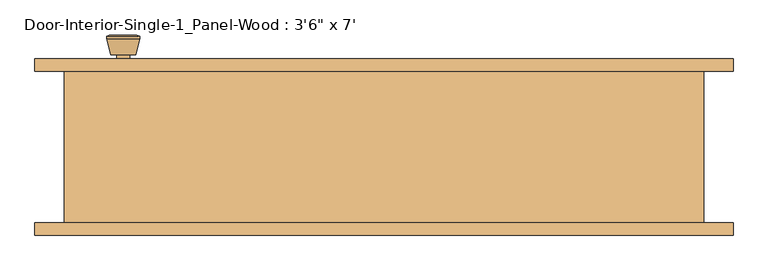
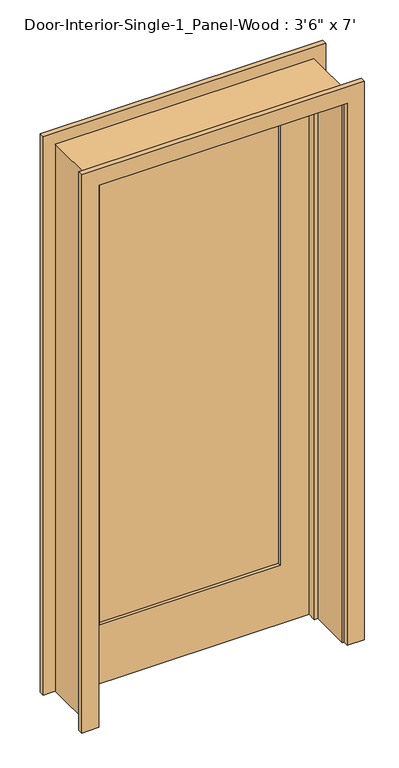
"""IFC4 building model written with IfcOpenShell, lengths in millimetres: door geometry."""

from ifc_helpers import new_model, si_unit, point, frame, frame_2d, origin, place, context, project, spatial, polyline, circle_curve, trimmed, segment, composite_curve, outline, extrude, faceted_brep, source, transform, mapped, element, save
from ifc_brep_helpers import plane_surface, cylinder_surface, revolved_surface, advanced_brep


def door_3b97b8e7(model_context):
    return source(origin(), model_context, "Body", "SolidModel", [
        advanced_brep(
        [(-393.7, 70.2, 914.4), (-383.7, 70.2, 914.4), (-403.7, 70.2, 914.4), (-373.2241324, 21.2, 914.4), (-393.7, 21.2, 914.4), (-414.1758676, 21.2, 914.4), (-368.7, 23.0278681, 914.4), (-418.7, 23.0278681, 914.4), (-368.7, 26.4915463, 914.4), (-418.7, 26.4915463, 914.4), (-375.063764, 51.2, 914.4), (-412.336236, 51.2, 914.4), (-383.7, 51.2, 914.4), (-403.7, 51.2, 914.4)],
        [
            (0, 1),
            (1, 2, circle_curve(frame((-393.7, 70.2, 914.4), z_axis=(0.0, 1.0, 0.0), x_axis=(-1.0, 0.0, 0.0)), 10.0)),
            (2, 0),
            (2, 1, circle_curve(frame((-393.7, 70.2, 914.4), z_axis=(0.0, 1.0, 0.0), x_axis=(-1.0, 0.0, 0.0)), 10.0)),
            (3, 4),
            (4, 5),
            (5, 3, circle_curve(frame((-393.7, 21.2, 914.4), z_axis=(0.0, -1.0, 0.0), x_axis=(-1.0, 0.0, 0.0)), 20.4758676)),
            (3, 5, circle_curve(frame((-393.7, 21.2, 914.4), z_axis=(0.0, -1.0, 0.0), x_axis=(-1.0, 0.0, 0.0)), 20.4758676)),
            (6, 3),
            (5, 7),
            (7, 6, circle_curve(frame((-393.7, 23.0278681, 914.4), z_axis=(0.0, -1.0, 0.0), x_axis=(-1.0, 0.0, 0.0)), 25.0)),
            (6, 7, circle_curve(frame((-393.7, 23.0278681, 914.4), z_axis=(0.0, -1.0, 0.0), x_axis=(-1.0, 0.0, 0.0)), 25.0)),
            (8, 6),
            (7, 9),
            (9, 8, circle_curve(frame((-393.7, 26.4915463, 914.4), z_axis=(0.0, -1.0, 0.0), x_axis=(-1.0, 0.0, 0.0)), 25.0)),
            (8, 9, circle_curve(frame((-393.7, 26.4915463, 914.4), z_axis=(0.0, -1.0, 0.0), x_axis=(-1.0, 0.0, 0.0)), 25.0)),
            (10, 8),
            (9, 11),
            (11, 10, circle_curve(frame((-393.7, 51.2, 914.4), z_axis=(0.0, -1.0, 0.0), x_axis=(-1.0, 0.0, 0.0)), 18.636236)),
            (10, 11, circle_curve(frame((-393.7, 51.2, 914.4), z_axis=(0.0, -1.0, 0.0), x_axis=(-1.0, 0.0, 0.0)), 18.636236)),
            (12, 10),
            (11, 13),
            (13, 12, circle_curve(frame((-393.7, 51.2, 914.4), z_axis=(0.0, -1.0, 0.0), x_axis=(-1.0, 0.0, 0.0)), 10.0)),
            (12, 13, circle_curve(frame((-393.7, 51.2, 914.4), z_axis=(0.0, -1.0, 0.0), x_axis=(-1.0, 0.0, 0.0)), 10.0)),
            (1, 12),
            (13, 2),
        ],
        [
            plane_surface(frame((-393.7, 70.2, 914.4), z_axis=(0.0, 1.0, 0.0), x_axis=(-1.0, 0.0, 0.0))),
            plane_surface(frame((-393.7, 21.2, 914.4), z_axis=(0.0, -1.0, 0.0), x_axis=(-1.0, 0.0, 0.0))),
            revolved_surface(polyline([(-414.1758676, 21.2, 914.4), (-418.7, 23.0278681, 914.4)]), (-393.7, 70.2, 914.4), (0.0, 1.0, 0.0)),
            cylinder_surface(frame((-393.7, 70.2, 914.4), z_axis=(0.0, 1.0, 0.0), x_axis=(-1.0, 0.0, 0.0)), 25.0),
            revolved_surface(polyline([(-418.7, 26.4915463, 914.4), (-412.336236, 51.2, 914.4)]), (-393.7, 70.2, 914.4), (0.0, 1.0, 0.0)),
            plane_surface(frame((-393.7, 51.2, 914.4), z_axis=(0.0, 1.0, 0.0), x_axis=(-1.0, 0.0, 0.0))),
            cylinder_surface(frame((-393.7, 70.2, 914.4), z_axis=(0.0, 1.0, 0.0), x_axis=(-1.0, 0.0, 0.0)), 10.0),
        ],
        [
            (0, [[1, 2, 3]]),
            (0, [[-3, 4, -1]]),
            (1, [[5, 6, 7]]),
            (1, [[-6, -5, 8]]),
            (2, [[9, -7, 10, 11]]),
            (2, [[-10, -8, -9, 12]]),
            (3, [[13, -11, 14, 15]]),
            (3, [[-14, -12, -13, 16]]),
            (4, [[17, -15, 18, 19]]),
            (4, [[-18, -16, -17, 20]]),
            (5, [[21, -19, 22, 23]]),
            (5, [[-22, -20, -21, 24]]),
            (6, [[25, -23, 26, -2]]),
            (6, [[-26, -24, -25, -4]]),
        ],
    ),
        extrude(outline(composite_curve([segment(trimmed(circle_curve(frame_2d((914.4, -393.7)), 30.0), [point((914.4, -423.7))], [point((914.4, -363.7))], False, "CARTESIAN"), True, "CONTINUOUS"), segment(trimmed(circle_curve(frame_2d((914.4, -393.7)), 30.0), [point((914.4, -363.7))], [point((914.4, -423.7))], False, "CARTESIAN"), True, "CONTINUOUS")], self_intersect=False)), frame((0.0, 70.2, 0.0), z_axis=(0.0, 1.0, 0.0), x_axis=(0.0, 0.0, 1.0)), (0.0, 0.0, 1.0), 6.0),
        advanced_brep(
        [(-393.7, 117.125, 914.4), (-403.7, 117.125, 914.4), (-383.7, 117.125, 914.4), (-373.2241324, 166.125, 914.4), (-414.1758676, 166.125, 914.4), (-393.7, 166.125, 914.4), (-368.7, 164.2971319, 914.4), (-418.7, 164.2971319, 914.4), (-368.7, 160.8334537, 914.4), (-418.7, 160.8334537, 914.4), (-375.063764, 136.125, 914.4), (-412.336236, 136.125, 914.4), (-383.7, 136.125, 914.4), (-403.7, 136.125, 914.4)],
        [
            (0, 1),
            (1, 2, circle_curve(frame((-393.7, 117.125, 914.4), z_axis=(0.0, -1.0, 0.0), x_axis=(-1.0, 0.0, 0.0)), 10.0)),
            (2, 0),
            (2, 1, circle_curve(frame((-393.7, 117.125, 914.4), z_axis=(0.0, -1.0, 0.0), x_axis=(-1.0, 0.0, 0.0)), 10.0)),
            (3, 4, circle_curve(frame((-393.7, 166.125, 914.4), z_axis=(0.0, 1.0, 0.0), x_axis=(-1.0, 0.0, 0.0)), 20.4758676)),
            (4, 5),
            (5, 3),
            (4, 3, circle_curve(frame((-393.7, 166.125, 914.4), z_axis=(0.0, 1.0, 0.0), x_axis=(-1.0, 0.0, 0.0)), 20.4758676)),
            (6, 7, circle_curve(frame((-393.7, 164.2971319, 914.4), z_axis=(0.0, 1.0, 0.0), x_axis=(-1.0, 0.0, 0.0)), 25.0)),
            (7, 4),
            (3, 6),
            (7, 6, circle_curve(frame((-393.7, 164.2971319, 914.4), z_axis=(0.0, 1.0, 0.0), x_axis=(-1.0, 0.0, 0.0)), 25.0)),
            (8, 9, circle_curve(frame((-393.7, 160.8334537, 914.4), z_axis=(0.0, 1.0, 0.0), x_axis=(-1.0, 0.0, 0.0)), 25.0)),
            (9, 7),
            (6, 8),
            (9, 8, circle_curve(frame((-393.7, 160.8334537, 914.4), z_axis=(0.0, 1.0, 0.0), x_axis=(-1.0, 0.0, 0.0)), 25.0)),
            (10, 11, circle_curve(frame((-393.7, 136.125, 914.4), z_axis=(0.0, 1.0, 0.0), x_axis=(-1.0, 0.0, 0.0)), 18.636236)),
            (11, 9),
            (8, 10),
            (11, 10, circle_curve(frame((-393.7, 136.125, 914.4), z_axis=(0.0, 1.0, 0.0), x_axis=(-1.0, 0.0, 0.0)), 18.636236)),
            (12, 13, circle_curve(frame((-393.7, 136.125, 914.4), z_axis=(0.0, 1.0, 0.0), x_axis=(-1.0, 0.0, 0.0)), 10.0)),
            (13, 11),
            (10, 12),
            (13, 12, circle_curve(frame((-393.7, 136.125, 914.4), z_axis=(0.0, 1.0, 0.0), x_axis=(-1.0, 0.0, 0.0)), 10.0)),
            (1, 13),
            (12, 2),
        ],
        [
            plane_surface(frame((-393.7, 117.125, 914.4), z_axis=(0.0, -1.0, 0.0), x_axis=(-1.0, 0.0, 0.0))),
            plane_surface(frame((-393.7, 166.125, 914.4), z_axis=(0.0, 1.0, 0.0), x_axis=(-1.0, 0.0, 0.0))),
            revolved_surface(polyline([(-414.1758676, 166.125, 914.4), (-418.7, 164.2971319, 914.4)]), (-393.7, 117.125, 914.4), (0.0, -1.0, 0.0)),
            cylinder_surface(frame((-393.7, 117.125, 914.4), z_axis=(0.0, -1.0, 0.0), x_axis=(-1.0, 0.0, 0.0)), 25.0),
            revolved_surface(polyline([(-418.7, 160.8334537, 914.4), (-412.336236, 136.125, 914.4)]), (-393.7, 117.125, 914.4), (0.0, -1.0, 0.0)),
            plane_surface(frame((-393.7, 136.125, 914.4), z_axis=(0.0, -1.0, 0.0), x_axis=(-1.0, 0.0, 0.0))),
            cylinder_surface(frame((-393.7, 117.125, 914.4), z_axis=(0.0, -1.0, 0.0), x_axis=(-1.0, 0.0, 0.0)), 10.0),
        ],
        [
            (0, [[1, 2, 3]]),
            (0, [[-3, 4, -1]]),
            (1, [[5, 6, 7]]),
            (1, [[8, -7, -6]]),
            (2, [[9, 10, -5, 11]]),
            (2, [[12, -11, -8, -10]]),
            (3, [[13, 14, -9, 15]]),
            (3, [[16, -15, -12, -14]]),
            (4, [[17, 18, -13, 19]]),
            (4, [[20, -19, -16, -18]]),
            (5, [[21, 22, -17, 23]]),
            (5, [[24, -23, -20, -22]]),
            (6, [[-2, 25, -21, 26]]),
            (6, [[-4, -26, -24, -25]]),
        ],
    ),
        extrude(outline(composite_curve([segment(trimmed(circle_curve(frame_2d((914.4, -393.7)), 30.0), [point((914.4, -423.7))], [point((914.4, -363.7))], False, "CARTESIAN"), True, "CONTINUOUS"), segment(trimmed(circle_curve(frame_2d((914.4, -393.7)), 30.0), [point((914.4, -363.7))], [point((914.4, -423.7))], False, "CARTESIAN"), True, "CONTINUOUS")], self_intersect=False)), frame((0.0, 111.125, 0.0), z_axis=(0.0, 1.0, 0.0), x_axis=(0.0, 0.0, 1.0)), (0.0, 0.0, 1.0), 6.0),
        faceted_brep([(482.6, 111.125, 0.0), (482.6, -117.475, 0.0), (457.2, -117.475, 0.0), (457.2, 41.275, 0.0), (444.5, 41.275, 0.0), (444.5, 76.2, 0.0), (457.2, 76.2, 0.0), (457.2, 111.125, 0.0), (482.6, 111.125, 2159.0), (482.6, -117.475, 2159.0), (-482.6, -117.475, 2159.0), (-482.6, -117.475, 0.0), (-457.2, -117.475, 0.0), (-457.2, -117.475, 2133.6), (457.2, -117.475, 2133.6), (457.2, 41.275, 2133.6), (-457.2, 41.275, 2133.6), (-457.2, 41.275, 0.0), (-444.5, 41.275, 0.0), (-444.5, 41.275, 2120.9), (444.5, 41.275, 2120.9), (444.5, 76.2, 2120.9), (-444.5, 76.2, 2120.9), (-444.5, 76.2, 0.0), (-457.2, 76.2, 0.0), (-457.2, 76.2, 2133.6), (457.2, 76.2, 2133.6), (457.2, 111.125, 2133.6), (-457.2, 111.125, 2133.6), (-457.2, 111.125, 0.0), (-482.6, 111.125, 0.0), (-482.6, 111.125, 2159.0)], [[[0, 1, 2, 3, 4, 5, 6, 7]], [[1, 0, 8, 9]], [[2, 1, 9, 10, 11, 12, 13, 14]], [[3, 2, 14, 15]], [[4, 3, 15, 16, 17, 18, 19, 20]], [[5, 4, 20, 21]], [[6, 5, 21, 22, 23, 24, 25, 26]], [[7, 6, 26, 27]], [[0, 7, 27, 28, 29, 30, 31, 8]], [[9, 8, 31, 10]], [[15, 14, 13, 16]], [[21, 20, 19, 22]], [[27, 26, 25, 28]], [[30, 29, 24, 23, 18, 17, 12, 11]], [[10, 31, 30, 11]], [[16, 13, 12, 17]], [[22, 19, 18, 23]], [[28, 25, 24, 29]]]),
        extrude(outline(polyline([(2133.6, -457.2), (0.0, -457.2), (0.0, 457.2), (2133.6, 457.2), (2133.6, -457.2)]), holes=[polyline([(2014.5375, -336.55), (2014.5375, 336.55), (231.775, 336.55), (231.775, -336.55), (2014.5375, -336.55)])]), frame((0.0, 76.2, 0.0), z_axis=(0.0, 1.0, 0.0), x_axis=(0.0, 0.0, 1.0)), (0.0, 0.0, 1.0), 34.925),
        extrude(outline(polyline([(336.55, 87.8416667), (-336.55, 87.8416667), (-336.55, 99.4833333), (336.55, 99.4833333), (336.55, 87.8416667)])), frame((0.0, 0.0, 231.775), z_axis=(0.0, 0.0, 1.0), x_axis=(1.0, 0.0, 0.0)), (0.0, 0.0, 1.0), 1782.7625),
        extrude(outline(polyline([(0.0, 463.55), (0.0, 527.05), (2203.45, 527.05), (2203.45, -527.05), (0.0, -527.05), (0.0, -463.55), (2139.95, -463.55), (2139.95, 463.55), (0.0, 463.55)])), frame((0.0, 111.125, 0.0), z_axis=(0.0, 1.0, 0.0), x_axis=(0.0, 0.0, 1.0)), (0.0, 0.0, 1.0), 19.05),
        extrude(outline(polyline([(0.0, 463.55), (0.0, 527.05), (2203.45, 527.05), (2203.45, -527.05), (0.0, -527.05), (0.0, -463.55), (2139.95, -463.55), (2139.95, 463.55), (0.0, 463.55)])), frame((0.0, -136.525, 0.0), z_axis=(0.0, 1.0, 0.0), x_axis=(0.0, 0.0, 1.0)), (0.0, 0.0, 1.0), 19.05),
    ])


if __name__ == "__main__":
    model = new_model("IFC4")
    model_context = context("Model", 3, world=origin())
    ifc_project = project(units=[si_unit("LENGTHUNIT", "METRE", prefix="MILLI")], contexts=[model_context])
    site = spatial("IfcSite", under=ifc_project)
    building = spatial("IfcBuilding", under=site)
    placement = place(None, origin())
    door_shape = door_3b97b8e7(model_context)
    element("IfcDoor", 1, ObjectType="Door-Interior-Single-1_Panel-Wood : 3'6\" x 7'", at=placement, inside=building, context=model_context, shape_type="MappedRepresentation", body=[
        mapped(door_shape, transform((0.0, 0.0, 0.0), x_axis=(1.0, 0.0, 0.0), y_axis=(0.0, 1.0, 0.0), z_axis=(0.0, 0.0, 1.0))),
    ])
    save(model, "model.ifc")

# Revit data of these elements
# Type "Door-Interior-Single-1_Panel-Wood : 3'6\" x 7'"
#   Type Mark = "9"
#   Assembly Code = "C1020300"
#   Analytic Construction = "Wooden"
#   Top Rail = 0' - 4 11/16"
#   Thickness = 0' - 1 3/8"
#   Thermal Resistance (R) = 2.5876 (h·ft²·°F)/BTU
#   Swing Angle [instance default] = 90.00°
#   Stiles = 0' - 4 3/4"
#   Rough Width = 3' - 2"
#   Rough Height = 7' - 1"
#   Height = 7' - 0"
#   Width = 3' - 0"
#   Heat Transfer Coefficient (U) = 0.3865 BTU/(h·ft²·°F)
#   Bottom Rail = 0' - 9 1/8"
#   Trim Material = door
#   Panel Material = door
#   Frame Material = door
#   Door Handle Material = Aluminum
#   Visual Light Transmittance = 0
#   Solar Heat Gain Coefficient = 0
#   Wall Closure = (empty or 0)
#   Function = (empty or 0)
# Element 1 (IfcDoor, "Door-Interior-Single-1_Panel-Wood : 3'6\" x 7'")
#   Materials on its faces: "door", "Aluminum"
# Materials
#   "door": class "Generic", colour RGB 120 120 120, transparency 0, Cost = 0
#   "Aluminum": class "Metal", colour RGB 247 247 247, transparency 0, Description = "Aluminum 6061", Cost = 0
